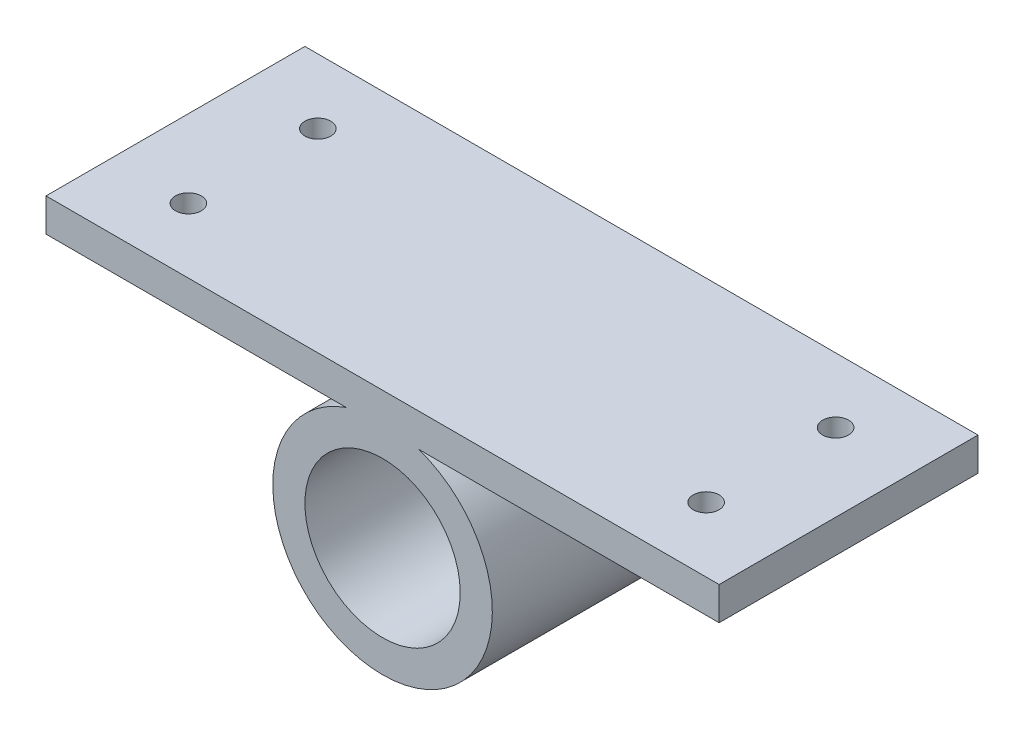
ISO-10303-21;
HEADER;
FILE_DESCRIPTION(('STEP AP214'),'2;1');
FILE_NAME('part.step','',(''),(''),'','','');
FILE_SCHEMA(('AUTOMOTIVE_DESIGN { 1 0 10303 214 1 1 1 1 }'));
ENDSEC;
DATA;
#1=APPLICATION_CONTEXT('core data for automotive mechanical design processes');
#2=APPLICATION_PROTOCOL_DEFINITION('international standard','automotive_design',2000,#1);
#3=PRODUCT_CONTEXT('',#1,'mechanical');
#4=PRODUCT('Part','Part','',(#3));
#5=PRODUCT_RELATED_PRODUCT_CATEGORY('part','',(#4));
#6=PRODUCT_DEFINITION_FORMATION('','',#4);
#7=PRODUCT_DEFINITION_CONTEXT('part definition',#1,'design');
#8=PRODUCT_DEFINITION('design','',#6,#7);
#9=PRODUCT_DEFINITION_SHAPE('','',#8);
#10=(LENGTH_UNIT() NAMED_UNIT(*) SI_UNIT(.MILLI.,.METRE.));
#11=(NAMED_UNIT(*) PLANE_ANGLE_UNIT() SI_UNIT($,.RADIAN.));
#12=(NAMED_UNIT(*) SI_UNIT($,.STERADIAN.) SOLID_ANGLE_UNIT());
#13=UNCERTAINTY_MEASURE_WITH_UNIT(LENGTH_MEASURE(1.E-05),#10,'distance_accuracy_value','');
#14=(GEOMETRIC_REPRESENTATION_CONTEXT(3) GLOBAL_UNCERTAINTY_ASSIGNED_CONTEXT((#13)) GLOBAL_UNIT_ASSIGNED_CONTEXT((#10,
#11,#12)) REPRESENTATION_CONTEXT('',''));
#15=CARTESIAN_POINT('',(0.,0.,0.));
#16=DIRECTION('',(0.,0.,1.));
#17=DIRECTION('',(1.,0.,0.));
#18=AXIS2_PLACEMENT_3D('',#15,#16,#17);
#19=CARTESIAN_POINT('',(0.,-116.,250.));
#20=DIRECTION('',(0.,0.,1.));
#21=DIRECTION('',(1.,0.,0.));
#22=AXIS2_PLACEMENT_3D('',#19,#20,#21);
#23=PLANE('',#22);
#24=DIRECTION('',(0.,1.,0.));
#25=VECTOR('',#24,1.);
#26=CARTESIAN_POINT('',(325.000000000001,-16.,250.));
#27=LINE('',#26,#25);
#28=CARTESIAN_POINT('',(325.000000000001,-16.,250.));
#29=VERTEX_POINT('',#28);
#30=CARTESIAN_POINT('',(325.000000000001,16.,250.));
#31=VERTEX_POINT('',#30);
#32=EDGE_CURVE('E131',#29,#31,#27,.T.);
#33=ORIENTED_EDGE('',*,*,#32,.T.);
#34=DIRECTION('',(-1.,0.,0.));
#35=VECTOR('',#34,1.);
#36=CARTESIAN_POINT('',(-324.999999999999,16.,250.));
#37=LINE('',#36,#35);
#38=CARTESIAN_POINT('',(-324.999999999999,16.,250.));
#39=VERTEX_POINT('',#38);
#40=EDGE_CURVE('E91',#31,#39,#37,.T.);
#41=ORIENTED_EDGE('',*,*,#40,.T.);
#42=DIRECTION('',(0.,-1.,0.));
#43=VECTOR('',#42,1.);
#44=CARTESIAN_POINT('',(-324.999999999999,-16.,250.));
#45=LINE('',#44,#43);
#46=CARTESIAN_POINT('',(-324.999999999999,-16.,250.));
#47=VERTEX_POINT('',#46);
#48=EDGE_CURVE('E106',#39,#47,#45,.T.);
#49=ORIENTED_EDGE('',*,*,#48,.T.);
#50=DIRECTION('',(1.,0.,0.));
#51=VECTOR('',#50,1.);
#52=CARTESIAN_POINT('',(-324.999999999999,-16.,250.));
#53=LINE('',#52,#51);
#54=CARTESIAN_POINT('',(-35.1567916624939,-16.,250.));
#55=VERTEX_POINT('',#54);
#56=EDGE_CURVE('E99',#47,#55,#53,.T.);
#57=ORIENTED_EDGE('',*,*,#56,.T.);
#58=CARTESIAN_POINT('',(0.,-116.,250.));
#59=DIRECTION('',(0.,0.,1.));
#60=DIRECTION('',(1.,0.,0.));
#61=AXIS2_PLACEMENT_3D('',#58,#59,#60);
#62=CIRCLE('',#61,106.);
#63=CARTESIAN_POINT('',(35.1567916624939,-16.,250.));
#64=VERTEX_POINT('',#63);
#65=EDGE_CURVE('E102',#55,#64,#62,.T.);
#66=ORIENTED_EDGE('',*,*,#65,.T.);
#67=DIRECTION('',(1.,0.,0.));
#68=VECTOR('',#67,1.);
#69=CARTESIAN_POINT('',(35.1567916624939,-16.,250.));
#70=LINE('',#69,#68);
#71=EDGE_CURVE('E57',#64,#29,#70,.T.);
#72=ORIENTED_EDGE('',*,*,#71,.T.);
#73=EDGE_LOOP('',(#33,#41,#49,#57,#66,#72));
#74=FACE_BOUND('',#73,.T.);
#75=CARTESIAN_POINT('',(0.,-116.,250.));
#76=DIRECTION('',(0.,0.,1.));
#77=DIRECTION('',(1.,0.,0.));
#78=AXIS2_PLACEMENT_3D('',#75,#76,#77);
#79=CIRCLE('',#78,75.);
#80=CARTESIAN_POINT('',(75.,-116.,250.));
#81=VERTEX_POINT('',#80);
#82=EDGE_CURVE('E126',#81,#81,#79,.T.);
#83=ORIENTED_EDGE('',*,*,#82,.F.);
#84=EDGE_LOOP('',(#83));
#85=FACE_BOUND('',#84,.T.);
#86=ADVANCED_FACE('F39',(#74,#85),#23,.T.);
#87=CARTESIAN_POINT('',(0.,-116.,0.));
#88=DIRECTION('',(0.,0.,1.));
#89=DIRECTION('',(1.,0.,0.));
#90=AXIS2_PLACEMENT_3D('',#87,#88,#89);
#91=PLANE('',#90);
#92=DIRECTION('',(0.,1.,0.));
#93=VECTOR('',#92,1.);
#94=CARTESIAN_POINT('',(325.000000000001,-16.,0.));
#95=LINE('',#94,#93);
#96=CARTESIAN_POINT('',(325.000000000001,-16.,0.));
#97=VERTEX_POINT('',#96);
#98=CARTESIAN_POINT('',(325.000000000001,16.,0.));
#99=VERTEX_POINT('',#98);
#100=EDGE_CURVE('E125',#97,#99,#95,.T.);
#101=ORIENTED_EDGE('',*,*,#100,.F.);
#102=DIRECTION('',(1.,0.,0.));
#103=VECTOR('',#102,1.);
#104=CARTESIAN_POINT('',(35.1567916624939,-16.,0.));
#105=LINE('',#104,#103);
#106=CARTESIAN_POINT('',(35.1567916624939,-16.,0.));
#107=VERTEX_POINT('',#106);
#108=EDGE_CURVE('E81',#107,#97,#105,.T.);
#109=ORIENTED_EDGE('',*,*,#108,.F.);
#110=CARTESIAN_POINT('',(0.,-116.,0.));
#111=DIRECTION('',(0.,0.,1.));
#112=DIRECTION('',(1.,0.,0.));
#113=AXIS2_PLACEMENT_3D('',#110,#111,#112);
#114=CIRCLE('',#113,106.);
#115=CARTESIAN_POINT('',(-35.1567916624939,-16.,0.));
#116=VERTEX_POINT('',#115);
#117=EDGE_CURVE('E80',#116,#107,#114,.T.);
#118=ORIENTED_EDGE('',*,*,#117,.F.);
#119=DIRECTION('',(1.,0.,0.));
#120=VECTOR('',#119,1.);
#121=CARTESIAN_POINT('',(-324.999999999999,-16.,0.));
#122=LINE('',#121,#120);
#123=CARTESIAN_POINT('',(-324.999999999999,-16.,0.));
#124=VERTEX_POINT('',#123);
#125=EDGE_CURVE('E111',#124,#116,#122,.T.);
#126=ORIENTED_EDGE('',*,*,#125,.F.);
#127=DIRECTION('',(0.,-1.,0.));
#128=VECTOR('',#127,1.);
#129=CARTESIAN_POINT('',(-324.999999999999,-16.,0.));
#130=LINE('',#129,#128);
#131=CARTESIAN_POINT('',(-324.999999999999,16.,0.));
#132=VERTEX_POINT('',#131);
#133=EDGE_CURVE('E128',#132,#124,#130,.T.);
#134=ORIENTED_EDGE('',*,*,#133,.F.);
#135=DIRECTION('',(-1.,0.,0.));
#136=VECTOR('',#135,1.);
#137=CARTESIAN_POINT('',(-324.999999999999,16.,0.));
#138=LINE('',#137,#136);
#139=EDGE_CURVE('E130',#99,#132,#138,.T.);
#140=ORIENTED_EDGE('',*,*,#139,.F.);
#141=EDGE_LOOP('',(#101,#109,#118,#126,#134,#140));
#142=FACE_BOUND('',#141,.T.);
#143=CARTESIAN_POINT('',(0.,-116.,0.));
#144=DIRECTION('',(0.,0.,1.));
#145=DIRECTION('',(1.,0.,0.));
#146=AXIS2_PLACEMENT_3D('',#143,#144,#145);
#147=CIRCLE('',#146,75.);
#148=CARTESIAN_POINT('',(75.,-116.,0.));
#149=VERTEX_POINT('',#148);
#150=EDGE_CURVE('E216',#149,#149,#147,.T.);
#151=ORIENTED_EDGE('',*,*,#150,.T.);
#152=EDGE_LOOP('',(#151));
#153=FACE_BOUND('',#152,.T.);
#154=ADVANCED_FACE('F145',(#142,#153),#91,.F.);
#155=CARTESIAN_POINT('',(325.000000000001,-16.,250.));
#156=DIRECTION('',(-1.,0.,0.));
#157=DIRECTION('',(0.,0.,1.));
#158=AXIS2_PLACEMENT_3D('',#155,#156,#157);
#159=PLANE('',#158);
#160=ORIENTED_EDGE('',*,*,#100,.T.);
#161=DIRECTION('',(0.,0.,-1.));
#162=VECTOR('',#161,1.);
#163=CARTESIAN_POINT('',(325.000000000001,16.,250.));
#164=LINE('',#163,#162);
#165=EDGE_CURVE('E11',#31,#99,#164,.T.);
#166=ORIENTED_EDGE('',*,*,#165,.F.);
#167=ORIENTED_EDGE('',*,*,#32,.F.);
#168=DIRECTION('',(0.,0.,-1.));
#169=VECTOR('',#168,1.);
#170=CARTESIAN_POINT('',(325.000000000001,-16.,250.));
#171=LINE('',#170,#169);
#172=EDGE_CURVE('E116',#29,#97,#171,.T.);
#173=ORIENTED_EDGE('',*,*,#172,.T.);
#174=EDGE_LOOP('',(#160,#166,#167,#173));
#175=FACE_BOUND('',#174,.T.);
#176=ADVANCED_FACE('F41',(#175),#159,.F.);
#177=CARTESIAN_POINT('',(-324.999999999999,16.,250.));
#178=DIRECTION('',(0.,-1.,0.));
#179=DIRECTION('',(0.,0.,-1.));
#180=AXIS2_PLACEMENT_3D('',#177,#178,#179);
#181=PLANE('',#180);
#182=CARTESIAN_POINT('',(249.999999999999,16.,62.5));
#183=DIRECTION('',(0.,1.,0.));
#184=DIRECTION('',(0.,0.,-1.));
#185=AXIS2_PLACEMENT_3D('',#182,#183,#184);
#186=CIRCLE('',#185,12.5);
#187=CARTESIAN_POINT('',(249.999999999999,16.,75.));
#188=VERTEX_POINT('',#187);
#189=EDGE_CURVE('E205',#188,#188,#186,.T.);
#190=ORIENTED_EDGE('',*,*,#189,.F.);
#191=EDGE_LOOP('',(#190));
#192=FACE_BOUND('',#191,.T.);
#193=CARTESIAN_POINT('',(-249.999999999999,16.,187.5));
#194=DIRECTION('',(0.,1.,0.));
#195=DIRECTION('',(0.,0.,1.));
#196=AXIS2_PLACEMENT_3D('',#193,#194,#195);
#197=CIRCLE('',#196,12.5);
#198=CARTESIAN_POINT('',(-249.999999999999,16.,200.));
#199=VERTEX_POINT('',#198);
#200=EDGE_CURVE('E191',#199,#199,#197,.T.);
#201=ORIENTED_EDGE('',*,*,#200,.F.);
#202=EDGE_LOOP('',(#201));
#203=FACE_BOUND('',#202,.T.);
#204=CARTESIAN_POINT('',(249.999999999999,16.,187.5));
#205=DIRECTION('',(0.,1.,0.));
#206=DIRECTION('',(0.,0.,-1.));
#207=AXIS2_PLACEMENT_3D('',#204,#205,#206);
#208=CIRCLE('',#207,12.5);
#209=CARTESIAN_POINT('',(249.999999999999,16.,200.));
#210=VERTEX_POINT('',#209);
#211=EDGE_CURVE('E193',#210,#210,#208,.T.);
#212=ORIENTED_EDGE('',*,*,#211,.F.);
#213=EDGE_LOOP('',(#212));
#214=FACE_BOUND('',#213,.T.);
#215=CARTESIAN_POINT('',(-249.999999999999,16.,62.5));
#216=DIRECTION('',(0.,1.,0.));
#217=DIRECTION('',(0.,0.,1.));
#218=AXIS2_PLACEMENT_3D('',#215,#216,#217);
#219=CIRCLE('',#218,12.5);
#220=CARTESIAN_POINT('',(-249.999999999999,16.,75.));
#221=VERTEX_POINT('',#220);
#222=EDGE_CURVE('E210',#221,#221,#219,.T.);
#223=ORIENTED_EDGE('',*,*,#222,.F.);
#224=EDGE_LOOP('',(#223));
#225=FACE_BOUND('',#224,.T.);
#226=ORIENTED_EDGE('',*,*,#139,.T.);
#227=DIRECTION('',(0.,0.,-1.));
#228=VECTOR('',#227,1.);
#229=CARTESIAN_POINT('',(-324.999999999999,16.,250.));
#230=LINE('',#229,#228);
#231=EDGE_CURVE('E48',#39,#132,#230,.T.);
#232=ORIENTED_EDGE('',*,*,#231,.F.);
#233=ORIENTED_EDGE('',*,*,#40,.F.);
#234=ORIENTED_EDGE('',*,*,#165,.T.);
#235=EDGE_LOOP('',(#226,#232,#233,#234));
#236=FACE_BOUND('',#235,.T.);
#237=ADVANCED_FACE('F235',(#192,#203,#214,#225,#236),#181,.F.);
#238=CARTESIAN_POINT('',(-324.999999999999,-16.,250.));
#239=DIRECTION('',(1.,0.,0.));
#240=DIRECTION('',(0.,0.,-1.));
#241=AXIS2_PLACEMENT_3D('',#238,#239,#240);
#242=PLANE('',#241);
#243=ORIENTED_EDGE('',*,*,#133,.T.);
#244=DIRECTION('',(0.,0.,-1.));
#245=VECTOR('',#244,1.);
#246=CARTESIAN_POINT('',(-324.999999999999,-16.,250.));
#247=LINE('',#246,#245);
#248=EDGE_CURVE('E113',#47,#124,#247,.T.);
#249=ORIENTED_EDGE('',*,*,#248,.F.);
#250=ORIENTED_EDGE('',*,*,#48,.F.);
#251=ORIENTED_EDGE('',*,*,#231,.T.);
#252=EDGE_LOOP('',(#243,#249,#250,#251));
#253=FACE_BOUND('',#252,.T.);
#254=ADVANCED_FACE('F143',(#253),#242,.F.);
#255=CARTESIAN_POINT('',(-324.999999999999,-16.,250.));
#256=DIRECTION('',(0.,1.,0.));
#257=DIRECTION('',(0.,0.,1.));
#258=AXIS2_PLACEMENT_3D('',#255,#256,#257);
#259=PLANE('',#258);
#260=CARTESIAN_POINT('',(-249.999999999999,-16.,187.5));
#261=DIRECTION('',(0.,1.,0.));
#262=DIRECTION('',(0.,0.,1.));
#263=AXIS2_PLACEMENT_3D('',#260,#261,#262);
#264=CIRCLE('',#263,12.5);
#265=CARTESIAN_POINT('',(-249.999999999999,-16.,200.));
#266=VERTEX_POINT('',#265);
#267=EDGE_CURVE('E196',#266,#266,#264,.F.);
#268=ORIENTED_EDGE('',*,*,#267,.F.);
#269=EDGE_LOOP('',(#268));
#270=FACE_BOUND('',#269,.T.);
#271=CARTESIAN_POINT('',(-249.999999999999,-16.,62.5));
#272=DIRECTION('',(0.,1.,0.));
#273=DIRECTION('',(0.,0.,1.));
#274=AXIS2_PLACEMENT_3D('',#271,#272,#273);
#275=CIRCLE('',#274,12.5);
#276=CARTESIAN_POINT('',(-249.999999999999,-16.,75.));
#277=VERTEX_POINT('',#276);
#278=EDGE_CURVE('E213',#277,#277,#275,.F.);
#279=ORIENTED_EDGE('',*,*,#278,.F.);
#280=EDGE_LOOP('',(#279));
#281=FACE_BOUND('',#280,.T.);
#282=ORIENTED_EDGE('',*,*,#125,.T.);
#283=DIRECTION('',(0.,0.,-1.));
#284=VECTOR('',#283,1.);
#285=CARTESIAN_POINT('',(-35.1567916624939,-16.,250.));
#286=LINE('',#285,#284);
#287=EDGE_CURVE('E112',#55,#116,#286,.T.);
#288=ORIENTED_EDGE('',*,*,#287,.F.);
#289=ORIENTED_EDGE('',*,*,#56,.F.);
#290=ORIENTED_EDGE('',*,*,#248,.T.);
#291=EDGE_LOOP('',(#282,#288,#289,#290));
#292=FACE_BOUND('',#291,.T.);
#293=ADVANCED_FACE('F115',(#270,#281,#292),#259,.F.);
#294=CARTESIAN_POINT('',(0.,-116.,250.));
#295=DIRECTION('',(0.,0.,-1.));
#296=DIRECTION('',(-1.,0.,0.));
#297=AXIS2_PLACEMENT_3D('',#294,#295,#296);
#298=CYLINDRICAL_SURFACE('',#297,106.);
#299=ORIENTED_EDGE('',*,*,#117,.T.);
#300=DIRECTION('',(0.,0.,-1.));
#301=VECTOR('',#300,1.);
#302=CARTESIAN_POINT('',(35.1567916624939,-16.,250.));
#303=LINE('',#302,#301);
#304=EDGE_CURVE('E118',#64,#107,#303,.T.);
#305=ORIENTED_EDGE('',*,*,#304,.F.);
#306=ORIENTED_EDGE('',*,*,#65,.F.);
#307=ORIENTED_EDGE('',*,*,#287,.T.);
#308=EDGE_LOOP('',(#299,#305,#306,#307));
#309=FACE_BOUND('',#308,.T.);
#310=ADVANCED_FACE('F117',(#309),#298,.T.);
#311=CARTESIAN_POINT('',(35.1567916624939,-16.,250.));
#312=DIRECTION('',(0.,1.,0.));
#313=DIRECTION('',(0.,0.,1.));
#314=AXIS2_PLACEMENT_3D('',#311,#312,#313);
#315=PLANE('',#314);
#316=CARTESIAN_POINT('',(249.999999999999,-16.,62.5));
#317=DIRECTION('',(0.,1.,0.));
#318=DIRECTION('',(0.,0.,1.));
#319=AXIS2_PLACEMENT_3D('',#316,#317,#318);
#320=CIRCLE('',#319,12.5);
#321=CARTESIAN_POINT('',(249.999999999999,-16.,75.));
#322=VERTEX_POINT('',#321);
#323=EDGE_CURVE('E202',#322,#322,#320,.F.);
#324=ORIENTED_EDGE('',*,*,#323,.F.);
#325=EDGE_LOOP('',(#324));
#326=FACE_BOUND('',#325,.T.);
#327=CARTESIAN_POINT('',(249.999999999999,-16.,187.5));
#328=DIRECTION('',(0.,1.,0.));
#329=DIRECTION('',(0.,0.,1.));
#330=AXIS2_PLACEMENT_3D('',#327,#328,#329);
#331=CIRCLE('',#330,12.5);
#332=CARTESIAN_POINT('',(249.999999999999,-16.,200.));
#333=VERTEX_POINT('',#332);
#334=EDGE_CURVE('E195',#333,#333,#331,.F.);
#335=ORIENTED_EDGE('',*,*,#334,.F.);
#336=EDGE_LOOP('',(#335));
#337=FACE_BOUND('',#336,.T.);
#338=ORIENTED_EDGE('',*,*,#108,.T.);
#339=ORIENTED_EDGE('',*,*,#172,.F.);
#340=ORIENTED_EDGE('',*,*,#71,.F.);
#341=ORIENTED_EDGE('',*,*,#304,.T.);
#342=EDGE_LOOP('',(#338,#339,#340,#341));
#343=FACE_BOUND('',#342,.T.);
#344=ADVANCED_FACE('F149',(#326,#337,#343),#315,.F.);
#345=CARTESIAN_POINT('',(0.,-116.,250.));
#346=DIRECTION('',(0.,0.,-1.));
#347=DIRECTION('',(-1.,0.,0.));
#348=AXIS2_PLACEMENT_3D('',#345,#346,#347);
#349=CYLINDRICAL_SURFACE('',#348,75.);
#350=ORIENTED_EDGE('',*,*,#82,.T.);
#351=EDGE_LOOP('',(#350));
#352=FACE_BOUND('',#351,.T.);
#353=ORIENTED_EDGE('',*,*,#150,.F.);
#354=EDGE_LOOP('',(#353));
#355=FACE_BOUND('',#354,.T.);
#356=ADVANCED_FACE('F151',(#352,#355),#349,.F.);
#357=CARTESIAN_POINT('',(249.999999999999,-222.001,187.5));
#358=DIRECTION('',(0.,1.,0.));
#359=DIRECTION('',(0.,0.,1.));
#360=AXIS2_PLACEMENT_3D('',#357,#358,#359);
#361=CYLINDRICAL_SURFACE('',#360,12.5);
#362=CARTESIAN_POINT('',(249.999999999999,16.,200.));
#363=CARTESIAN_POINT('',(249.999999999999,15.6666666666667,200.));
#364=CARTESIAN_POINT('',(249.999999999999,15.3333333333333,200.));
#365=CARTESIAN_POINT('',(249.999999999999,14.6666666666667,200.));
#366=CARTESIAN_POINT('',(249.999999999999,14.3333333333333,200.));
#367=CARTESIAN_POINT('',(249.999999999999,13.6666666666667,200.));
#368=CARTESIAN_POINT('',(249.999999999999,13.3333333333333,200.));
#369=CARTESIAN_POINT('',(249.999999999999,12.6666666666667,200.));
#370=CARTESIAN_POINT('',(249.999999999999,12.3333333333333,200.));
#371=CARTESIAN_POINT('',(249.999999999999,11.6666666666667,200.));
#372=CARTESIAN_POINT('',(249.999999999999,11.3333333333333,200.));
#373=CARTESIAN_POINT('',(249.999999999999,10.6666666666666,200.));
#374=CARTESIAN_POINT('',(249.999999999999,10.3333333333333,200.));
#375=CARTESIAN_POINT('',(249.999999999999,9.66666666666665,200.));
#376=CARTESIAN_POINT('',(249.999999999999,9.33333333333331,200.));
#377=CARTESIAN_POINT('',(249.999999999999,8.66666666666665,200.));
#378=CARTESIAN_POINT('',(249.999999999999,8.33333333333331,200.));
#379=CARTESIAN_POINT('',(249.999999999999,7.66666666666665,200.));
#380=CARTESIAN_POINT('',(249.999999999999,7.33333333333331,200.));
#381=CARTESIAN_POINT('',(249.999999999999,6.66666666666664,200.));
#382=CARTESIAN_POINT('',(249.999999999999,6.33333333333331,200.));
#383=CARTESIAN_POINT('',(249.999999999999,5.66666666666664,200.));
#384=CARTESIAN_POINT('',(249.999999999999,5.33333333333331,200.));
#385=CARTESIAN_POINT('',(249.999999999999,4.66666666666664,200.));
#386=CARTESIAN_POINT('',(249.999999999999,4.33333333333331,200.));
#387=CARTESIAN_POINT('',(249.999999999999,3.66666666666664,200.));
#388=CARTESIAN_POINT('',(249.999999999999,3.33333333333331,200.));
#389=CARTESIAN_POINT('',(249.999999999999,2.66666666666664,200.));
#390=CARTESIAN_POINT('',(249.999999999999,2.33333333333331,200.));
#391=CARTESIAN_POINT('',(249.999999999999,1.66666666666664,200.));
#392=CARTESIAN_POINT('',(249.999999999999,1.33333333333331,200.));
#393=CARTESIAN_POINT('',(249.999999999999,0.666666666666639,200.));
#394=CARTESIAN_POINT('',(249.999999999999,0.333333333333306,200.));
#395=CARTESIAN_POINT('',(249.999999999999,-0.333333333333361,200.));
#396=CARTESIAN_POINT('',(249.999999999999,-0.666666666666695,200.));
#397=CARTESIAN_POINT('',(249.999999999999,-1.33333333333336,200.));
#398=CARTESIAN_POINT('',(249.999999999999,-1.6666666666667,200.));
#399=CARTESIAN_POINT('',(249.999999999999,-2.33333333333336,200.));
#400=CARTESIAN_POINT('',(249.999999999999,-2.6666666666667,200.));
#401=CARTESIAN_POINT('',(249.999999999999,-3.33333333333336,200.));
#402=CARTESIAN_POINT('',(249.999999999999,-3.6666666666667,200.));
#403=CARTESIAN_POINT('',(249.999999999999,-4.33333333333337,200.));
#404=CARTESIAN_POINT('',(249.999999999999,-4.6666666666667,200.));
#405=CARTESIAN_POINT('',(249.999999999999,-5.33333333333337,200.));
#406=CARTESIAN_POINT('',(249.999999999999,-5.6666666666667,200.));
#407=CARTESIAN_POINT('',(249.999999999999,-6.33333333333337,200.));
#408=CARTESIAN_POINT('',(249.999999999999,-6.6666666666667,200.));
#409=CARTESIAN_POINT('',(249.999999999999,-7.33333333333337,200.));
#410=CARTESIAN_POINT('',(249.999999999999,-7.6666666666667,200.));
#411=CARTESIAN_POINT('',(249.999999999999,-8.33333333333337,200.));
#412=CARTESIAN_POINT('',(249.999999999999,-8.6666666666667,200.));
#413=CARTESIAN_POINT('',(249.999999999999,-9.33333333333337,200.));
#414=CARTESIAN_POINT('',(249.999999999999,-9.6666666666667,200.));
#415=CARTESIAN_POINT('',(249.999999999999,-10.3333333333334,200.));
#416=CARTESIAN_POINT('',(249.999999999999,-10.6666666666667,200.));
#417=CARTESIAN_POINT('',(249.999999999999,-11.3333333333334,200.));
#418=CARTESIAN_POINT('',(249.999999999999,-11.6666666666667,200.));
#419=CARTESIAN_POINT('',(249.999999999999,-12.3333333333334,200.));
#420=CARTESIAN_POINT('',(249.999999999999,-12.6666666666667,200.));
#421=CARTESIAN_POINT('',(249.999999999999,-13.3333333333334,200.));
#422=CARTESIAN_POINT('',(249.999999999999,-13.6666666666667,200.));
#423=CARTESIAN_POINT('',(249.999999999999,-14.3333333333334,200.));
#424=CARTESIAN_POINT('',(249.999999999999,-14.6666666666667,200.));
#425=CARTESIAN_POINT('',(249.999999999999,-15.3333333333334,200.));
#426=CARTESIAN_POINT('',(249.999999999999,-15.6666666666667,200.));
#427=CARTESIAN_POINT('',(249.999999999999,-16.,200.));
#428=B_SPLINE_CURVE_WITH_KNOTS('',3,(#362,#363,#364,#365,#366,#367,#368,#369,#370,#371,#372,
#373,#374,#375,#376,#377,#378,#379,#380,#381,#382,#383,#384,#385,#386,#387,#388,#389,#390,#391,
#392,#393,#394,#395,#396,#397,#398,#399,#400,#401,#402,#403,#404,#405,#406,#407,#408,#409,#410,
#411,#412,#413,#414,#415,#416,#417,#418,#419,#420,#421,#422,#423,#424,#425,#426,#427),
.UNSPECIFIED.,.F.,.F.,(4,2,2,2,2,2,2,2,2,2,2,2,2,2,2,2,2,2,2,2,2,2,2,2,2,2,2,2,2,2,2,2,4),(0.,
1.,2.,3.,4.,5.,6.00000000000001,7.00000000000001,8.00000000000001,9.00000000000001,10.,11.,12.,
13.,14.,15.,16.,17.,18.,19.,20.,21.,22.,23.,24.,25.,26.,27.,28.,29.,30.,31.,32.),.UNSPECIFIED.);
#429=EDGE_CURVE('BSEAM157',#210,#333,#428,.T.);
#430=ORIENTED_EDGE('',*,*,#211,.T.);
#431=ORIENTED_EDGE('',*,*,#334,.T.);
#432=ORIENTED_EDGE('',*,*,#429,.T.);
#433=ORIENTED_EDGE('',*,*,#429,.F.);
#434=EDGE_LOOP('',(#430,#432,#431,#433));
#435=FACE_BOUND('',#434,.T.);
#436=ADVANCED_FACE('F157',(#435),#361,.F.);
#437=CARTESIAN_POINT('',(249.999999999999,-222.001,62.5));
#438=DIRECTION('',(0.,1.,0.));
#439=DIRECTION('',(0.,0.,1.));
#440=AXIS2_PLACEMENT_3D('',#437,#438,#439);
#441=CYLINDRICAL_SURFACE('',#440,12.5);
#442=CARTESIAN_POINT('',(249.999999999999,16.,75.));
#443=CARTESIAN_POINT('',(249.999999999999,15.6666666666667,75.));
#444=CARTESIAN_POINT('',(249.999999999999,15.3333333333333,75.));
#445=CARTESIAN_POINT('',(249.999999999999,14.6666666666667,75.));
#446=CARTESIAN_POINT('',(249.999999999999,14.3333333333333,75.));
#447=CARTESIAN_POINT('',(249.999999999999,13.6666666666667,75.));
#448=CARTESIAN_POINT('',(249.999999999999,13.3333333333333,75.));
#449=CARTESIAN_POINT('',(249.999999999999,12.6666666666667,75.));
#450=CARTESIAN_POINT('',(249.999999999999,12.3333333333333,75.));
#451=CARTESIAN_POINT('',(249.999999999999,11.6666666666667,75.));
#452=CARTESIAN_POINT('',(249.999999999999,11.3333333333333,75.));
#453=CARTESIAN_POINT('',(249.999999999999,10.6666666666666,75.));
#454=CARTESIAN_POINT('',(249.999999999999,10.3333333333333,75.));
#455=CARTESIAN_POINT('',(249.999999999999,9.66666666666665,75.));
#456=CARTESIAN_POINT('',(249.999999999999,9.33333333333331,75.));
#457=CARTESIAN_POINT('',(249.999999999999,8.66666666666665,75.));
#458=CARTESIAN_POINT('',(249.999999999999,8.33333333333331,75.));
#459=CARTESIAN_POINT('',(249.999999999999,7.66666666666665,75.));
#460=CARTESIAN_POINT('',(249.999999999999,7.33333333333331,75.));
#461=CARTESIAN_POINT('',(249.999999999999,6.66666666666664,75.));
#462=CARTESIAN_POINT('',(249.999999999999,6.33333333333331,75.));
#463=CARTESIAN_POINT('',(249.999999999999,5.66666666666664,75.));
#464=CARTESIAN_POINT('',(249.999999999999,5.33333333333331,75.));
#465=CARTESIAN_POINT('',(249.999999999999,4.66666666666664,75.));
#466=CARTESIAN_POINT('',(249.999999999999,4.33333333333331,75.));
#467=CARTESIAN_POINT('',(249.999999999999,3.66666666666664,75.));
#468=CARTESIAN_POINT('',(249.999999999999,3.33333333333331,75.));
#469=CARTESIAN_POINT('',(249.999999999999,2.66666666666664,75.));
#470=CARTESIAN_POINT('',(249.999999999999,2.33333333333331,75.));
#471=CARTESIAN_POINT('',(249.999999999999,1.66666666666664,75.));
#472=CARTESIAN_POINT('',(249.999999999999,1.33333333333331,75.));
#473=CARTESIAN_POINT('',(249.999999999999,0.666666666666639,75.));
#474=CARTESIAN_POINT('',(249.999999999999,0.333333333333306,75.));
#475=CARTESIAN_POINT('',(249.999999999999,-0.333333333333361,75.));
#476=CARTESIAN_POINT('',(249.999999999999,-0.666666666666695,75.));
#477=CARTESIAN_POINT('',(249.999999999999,-1.33333333333336,75.));
#478=CARTESIAN_POINT('',(249.999999999999,-1.6666666666667,75.));
#479=CARTESIAN_POINT('',(249.999999999999,-2.33333333333336,75.));
#480=CARTESIAN_POINT('',(249.999999999999,-2.6666666666667,75.));
#481=CARTESIAN_POINT('',(249.999999999999,-3.33333333333336,75.));
#482=CARTESIAN_POINT('',(249.999999999999,-3.6666666666667,75.));
#483=CARTESIAN_POINT('',(249.999999999999,-4.33333333333337,75.));
#484=CARTESIAN_POINT('',(249.999999999999,-4.6666666666667,75.));
#485=CARTESIAN_POINT('',(249.999999999999,-5.33333333333337,75.));
#486=CARTESIAN_POINT('',(249.999999999999,-5.6666666666667,75.));
#487=CARTESIAN_POINT('',(249.999999999999,-6.33333333333337,75.));
#488=CARTESIAN_POINT('',(249.999999999999,-6.6666666666667,75.));
#489=CARTESIAN_POINT('',(249.999999999999,-7.33333333333337,75.));
#490=CARTESIAN_POINT('',(249.999999999999,-7.6666666666667,75.));
#491=CARTESIAN_POINT('',(249.999999999999,-8.33333333333337,75.));
#492=CARTESIAN_POINT('',(249.999999999999,-8.6666666666667,75.));
#493=CARTESIAN_POINT('',(249.999999999999,-9.33333333333337,75.));
#494=CARTESIAN_POINT('',(249.999999999999,-9.6666666666667,75.));
#495=CARTESIAN_POINT('',(249.999999999999,-10.3333333333334,75.));
#496=CARTESIAN_POINT('',(249.999999999999,-10.6666666666667,75.));
#497=CARTESIAN_POINT('',(249.999999999999,-11.3333333333334,75.));
#498=CARTESIAN_POINT('',(249.999999999999,-11.6666666666667,75.));
#499=CARTESIAN_POINT('',(249.999999999999,-12.3333333333334,75.));
#500=CARTESIAN_POINT('',(249.999999999999,-12.6666666666667,75.));
#501=CARTESIAN_POINT('',(249.999999999999,-13.3333333333334,75.));
#502=CARTESIAN_POINT('',(249.999999999999,-13.6666666666667,75.));
#503=CARTESIAN_POINT('',(249.999999999999,-14.3333333333334,75.));
#504=CARTESIAN_POINT('',(249.999999999999,-14.6666666666667,75.));
#505=CARTESIAN_POINT('',(249.999999999999,-15.3333333333334,75.));
#506=CARTESIAN_POINT('',(249.999999999999,-15.6666666666667,75.));
#507=CARTESIAN_POINT('',(249.999999999999,-16.,75.));
#508=B_SPLINE_CURVE_WITH_KNOTS('',3,(#442,#443,#444,#445,#446,#447,#448,#449,#450,#451,#452,
#453,#454,#455,#456,#457,#458,#459,#460,#461,#462,#463,#464,#465,#466,#467,#468,#469,#470,#471,
#472,#473,#474,#475,#476,#477,#478,#479,#480,#481,#482,#483,#484,#485,#486,#487,#488,#489,#490,
#491,#492,#493,#494,#495,#496,#497,#498,#499,#500,#501,#502,#503,#504,#505,#506,#507),
.UNSPECIFIED.,.F.,.F.,(4,2,2,2,2,2,2,2,2,2,2,2,2,2,2,2,2,2,2,2,2,2,2,2,2,2,2,2,2,2,2,2,4),(0.,
1.,2.,3.,4.,5.,6.00000000000001,7.00000000000001,8.00000000000001,9.00000000000001,10.,11.,12.,
13.,14.,15.,16.,17.,18.,19.,20.,21.,22.,23.,24.,25.,26.,27.,28.,29.,30.,31.,32.),.UNSPECIFIED.);
#509=EDGE_CURVE('BSEAM179',#188,#322,#508,.T.);
#510=ORIENTED_EDGE('',*,*,#189,.T.);
#511=ORIENTED_EDGE('',*,*,#323,.T.);
#512=ORIENTED_EDGE('',*,*,#509,.T.);
#513=ORIENTED_EDGE('',*,*,#509,.F.);
#514=EDGE_LOOP('',(#510,#512,#511,#513));
#515=FACE_BOUND('',#514,.T.);
#516=ADVANCED_FACE('F179',(#515),#441,.F.);
#517=CARTESIAN_POINT('',(-249.999999999999,-222.001,62.5));
#518=DIRECTION('',(0.,1.,0.));
#519=DIRECTION('',(0.,0.,1.));
#520=AXIS2_PLACEMENT_3D('',#517,#518,#519);
#521=CYLINDRICAL_SURFACE('',#520,12.5);
#522=CARTESIAN_POINT('',(-249.999999999999,16.,75.));
#523=CARTESIAN_POINT('',(-249.999999999999,15.6666666666667,75.));
#524=CARTESIAN_POINT('',(-249.999999999999,15.3333333333333,75.));
#525=CARTESIAN_POINT('',(-249.999999999999,14.6666666666667,75.));
#526=CARTESIAN_POINT('',(-249.999999999999,14.3333333333333,75.));
#527=CARTESIAN_POINT('',(-249.999999999999,13.6666666666667,75.));
#528=CARTESIAN_POINT('',(-249.999999999999,13.3333333333333,75.));
#529=CARTESIAN_POINT('',(-249.999999999999,12.6666666666667,75.));
#530=CARTESIAN_POINT('',(-249.999999999999,12.3333333333333,75.));
#531=CARTESIAN_POINT('',(-249.999999999999,11.6666666666667,75.));
#532=CARTESIAN_POINT('',(-249.999999999999,11.3333333333333,75.));
#533=CARTESIAN_POINT('',(-249.999999999999,10.6666666666666,75.));
#534=CARTESIAN_POINT('',(-249.999999999999,10.3333333333333,75.));
#535=CARTESIAN_POINT('',(-249.999999999999,9.66666666666665,75.));
#536=CARTESIAN_POINT('',(-249.999999999999,9.33333333333331,75.));
#537=CARTESIAN_POINT('',(-249.999999999999,8.66666666666665,75.));
#538=CARTESIAN_POINT('',(-249.999999999999,8.33333333333331,75.));
#539=CARTESIAN_POINT('',(-249.999999999999,7.66666666666665,75.));
#540=CARTESIAN_POINT('',(-249.999999999999,7.33333333333331,75.));
#541=CARTESIAN_POINT('',(-249.999999999999,6.66666666666664,75.));
#542=CARTESIAN_POINT('',(-249.999999999999,6.33333333333331,75.));
#543=CARTESIAN_POINT('',(-249.999999999999,5.66666666666664,75.));
#544=CARTESIAN_POINT('',(-249.999999999999,5.33333333333331,75.));
#545=CARTESIAN_POINT('',(-249.999999999999,4.66666666666664,75.));
#546=CARTESIAN_POINT('',(-249.999999999999,4.33333333333331,75.));
#547=CARTESIAN_POINT('',(-249.999999999999,3.66666666666664,75.));
#548=CARTESIAN_POINT('',(-249.999999999999,3.33333333333331,75.));
#549=CARTESIAN_POINT('',(-249.999999999999,2.66666666666664,75.));
#550=CARTESIAN_POINT('',(-249.999999999999,2.33333333333331,75.));
#551=CARTESIAN_POINT('',(-249.999999999999,1.66666666666664,75.));
#552=CARTESIAN_POINT('',(-249.999999999999,1.33333333333331,75.));
#553=CARTESIAN_POINT('',(-249.999999999999,0.666666666666639,75.));
#554=CARTESIAN_POINT('',(-249.999999999999,0.333333333333306,75.));
#555=CARTESIAN_POINT('',(-249.999999999999,-0.333333333333361,75.));
#556=CARTESIAN_POINT('',(-249.999999999999,-0.666666666666695,75.));
#557=CARTESIAN_POINT('',(-249.999999999999,-1.33333333333336,75.));
#558=CARTESIAN_POINT('',(-249.999999999999,-1.6666666666667,75.));
#559=CARTESIAN_POINT('',(-249.999999999999,-2.33333333333336,75.));
#560=CARTESIAN_POINT('',(-249.999999999999,-2.6666666666667,75.));
#561=CARTESIAN_POINT('',(-249.999999999999,-3.33333333333336,75.));
#562=CARTESIAN_POINT('',(-249.999999999999,-3.6666666666667,75.));
#563=CARTESIAN_POINT('',(-249.999999999999,-4.33333333333337,75.));
#564=CARTESIAN_POINT('',(-249.999999999999,-4.6666666666667,75.));
#565=CARTESIAN_POINT('',(-249.999999999999,-5.33333333333337,75.));
#566=CARTESIAN_POINT('',(-249.999999999999,-5.6666666666667,75.));
#567=CARTESIAN_POINT('',(-249.999999999999,-6.33333333333337,75.));
#568=CARTESIAN_POINT('',(-249.999999999999,-6.6666666666667,75.));
#569=CARTESIAN_POINT('',(-249.999999999999,-7.33333333333337,75.));
#570=CARTESIAN_POINT('',(-249.999999999999,-7.6666666666667,75.));
#571=CARTESIAN_POINT('',(-249.999999999999,-8.33333333333337,75.));
#572=CARTESIAN_POINT('',(-249.999999999999,-8.6666666666667,75.));
#573=CARTESIAN_POINT('',(-249.999999999999,-9.33333333333337,75.));
#574=CARTESIAN_POINT('',(-249.999999999999,-9.6666666666667,75.));
#575=CARTESIAN_POINT('',(-249.999999999999,-10.3333333333334,75.));
#576=CARTESIAN_POINT('',(-249.999999999999,-10.6666666666667,75.));
#577=CARTESIAN_POINT('',(-249.999999999999,-11.3333333333334,75.));
#578=CARTESIAN_POINT('',(-249.999999999999,-11.6666666666667,75.));
#579=CARTESIAN_POINT('',(-249.999999999999,-12.3333333333334,75.));
#580=CARTESIAN_POINT('',(-249.999999999999,-12.6666666666667,75.));
#581=CARTESIAN_POINT('',(-249.999999999999,-13.3333333333334,75.));
#582=CARTESIAN_POINT('',(-249.999999999999,-13.6666666666667,75.));
#583=CARTESIAN_POINT('',(-249.999999999999,-14.3333333333334,75.));
#584=CARTESIAN_POINT('',(-249.999999999999,-14.6666666666667,75.));
#585=CARTESIAN_POINT('',(-249.999999999999,-15.3333333333334,75.));
#586=CARTESIAN_POINT('',(-249.999999999999,-15.6666666666667,75.));
#587=CARTESIAN_POINT('',(-249.999999999999,-16.,75.));
#588=B_SPLINE_CURVE_WITH_KNOTS('',3,(#522,#523,#524,#525,#526,#527,#528,#529,#530,#531,#532,
#533,#534,#535,#536,#537,#538,#539,#540,#541,#542,#543,#544,#545,#546,#547,#548,#549,#550,#551,
#552,#553,#554,#555,#556,#557,#558,#559,#560,#561,#562,#563,#564,#565,#566,#567,#568,#569,#570,
#571,#572,#573,#574,#575,#576,#577,#578,#579,#580,#581,#582,#583,#584,#585,#586,#587),
.UNSPECIFIED.,.F.,.F.,(4,2,2,2,2,2,2,2,2,2,2,2,2,2,2,2,2,2,2,2,2,2,2,2,2,2,2,2,2,2,2,2,4),(0.,
1.,2.,3.,4.,5.,6.00000000000001,7.00000000000001,8.00000000000001,9.00000000000001,10.,11.,12.,
13.,14.,15.,16.,17.,18.,19.,20.,21.,22.,23.,24.,25.,26.,27.,28.,29.,30.,31.,32.),.UNSPECIFIED.);
#589=EDGE_CURVE('BSEAM172',#221,#277,#588,.T.);
#590=ORIENTED_EDGE('',*,*,#222,.T.);
#591=ORIENTED_EDGE('',*,*,#278,.T.);
#592=ORIENTED_EDGE('',*,*,#589,.T.);
#593=ORIENTED_EDGE('',*,*,#589,.F.);
#594=EDGE_LOOP('',(#590,#592,#591,#593));
#595=FACE_BOUND('',#594,.T.);
#596=ADVANCED_FACE('F172',(#595),#521,.F.);
#597=CARTESIAN_POINT('',(-249.999999999999,-222.001,187.5));
#598=DIRECTION('',(0.,1.,0.));
#599=DIRECTION('',(0.,0.,1.));
#600=AXIS2_PLACEMENT_3D('',#597,#598,#599);
#601=CYLINDRICAL_SURFACE('',#600,12.5);
#602=CARTESIAN_POINT('',(-249.999999999999,16.,200.));
#603=CARTESIAN_POINT('',(-249.999999999999,15.6666666666667,200.));
#604=CARTESIAN_POINT('',(-249.999999999999,15.3333333333333,200.));
#605=CARTESIAN_POINT('',(-249.999999999999,14.6666666666667,200.));
#606=CARTESIAN_POINT('',(-249.999999999999,14.3333333333333,200.));
#607=CARTESIAN_POINT('',(-249.999999999999,13.6666666666667,200.));
#608=CARTESIAN_POINT('',(-249.999999999999,13.3333333333333,200.));
#609=CARTESIAN_POINT('',(-249.999999999999,12.6666666666667,200.));
#610=CARTESIAN_POINT('',(-249.999999999999,12.3333333333333,200.));
#611=CARTESIAN_POINT('',(-249.999999999999,11.6666666666667,200.));
#612=CARTESIAN_POINT('',(-249.999999999999,11.3333333333333,200.));
#613=CARTESIAN_POINT('',(-249.999999999999,10.6666666666666,200.));
#614=CARTESIAN_POINT('',(-249.999999999999,10.3333333333333,200.));
#615=CARTESIAN_POINT('',(-249.999999999999,9.66666666666665,200.));
#616=CARTESIAN_POINT('',(-249.999999999999,9.33333333333331,200.));
#617=CARTESIAN_POINT('',(-249.999999999999,8.66666666666665,200.));
#618=CARTESIAN_POINT('',(-249.999999999999,8.33333333333331,200.));
#619=CARTESIAN_POINT('',(-249.999999999999,7.66666666666665,200.));
#620=CARTESIAN_POINT('',(-249.999999999999,7.33333333333331,200.));
#621=CARTESIAN_POINT('',(-249.999999999999,6.66666666666664,200.));
#622=CARTESIAN_POINT('',(-249.999999999999,6.33333333333331,200.));
#623=CARTESIAN_POINT('',(-249.999999999999,5.66666666666664,200.));
#624=CARTESIAN_POINT('',(-249.999999999999,5.33333333333331,200.));
#625=CARTESIAN_POINT('',(-249.999999999999,4.66666666666664,200.));
#626=CARTESIAN_POINT('',(-249.999999999999,4.33333333333331,200.));
#627=CARTESIAN_POINT('',(-249.999999999999,3.66666666666664,200.));
#628=CARTESIAN_POINT('',(-249.999999999999,3.33333333333331,200.));
#629=CARTESIAN_POINT('',(-249.999999999999,2.66666666666664,200.));
#630=CARTESIAN_POINT('',(-249.999999999999,2.33333333333331,200.));
#631=CARTESIAN_POINT('',(-249.999999999999,1.66666666666664,200.));
#632=CARTESIAN_POINT('',(-249.999999999999,1.33333333333331,200.));
#633=CARTESIAN_POINT('',(-249.999999999999,0.666666666666639,200.));
#634=CARTESIAN_POINT('',(-249.999999999999,0.333333333333306,200.));
#635=CARTESIAN_POINT('',(-249.999999999999,-0.333333333333361,200.));
#636=CARTESIAN_POINT('',(-249.999999999999,-0.666666666666695,200.));
#637=CARTESIAN_POINT('',(-249.999999999999,-1.33333333333336,200.));
#638=CARTESIAN_POINT('',(-249.999999999999,-1.6666666666667,200.));
#639=CARTESIAN_POINT('',(-249.999999999999,-2.33333333333336,200.));
#640=CARTESIAN_POINT('',(-249.999999999999,-2.6666666666667,200.));
#641=CARTESIAN_POINT('',(-249.999999999999,-3.33333333333336,200.));
#642=CARTESIAN_POINT('',(-249.999999999999,-3.6666666666667,200.));
#643=CARTESIAN_POINT('',(-249.999999999999,-4.33333333333337,200.));
#644=CARTESIAN_POINT('',(-249.999999999999,-4.6666666666667,200.));
#645=CARTESIAN_POINT('',(-249.999999999999,-5.33333333333337,200.));
#646=CARTESIAN_POINT('',(-249.999999999999,-5.6666666666667,200.));
#647=CARTESIAN_POINT('',(-249.999999999999,-6.33333333333337,200.));
#648=CARTESIAN_POINT('',(-249.999999999999,-6.6666666666667,200.));
#649=CARTESIAN_POINT('',(-249.999999999999,-7.33333333333337,200.));
#650=CARTESIAN_POINT('',(-249.999999999999,-7.6666666666667,200.));
#651=CARTESIAN_POINT('',(-249.999999999999,-8.33333333333337,200.));
#652=CARTESIAN_POINT('',(-249.999999999999,-8.6666666666667,200.));
#653=CARTESIAN_POINT('',(-249.999999999999,-9.33333333333337,200.));
#654=CARTESIAN_POINT('',(-249.999999999999,-9.6666666666667,200.));
#655=CARTESIAN_POINT('',(-249.999999999999,-10.3333333333334,200.));
#656=CARTESIAN_POINT('',(-249.999999999999,-10.6666666666667,200.));
#657=CARTESIAN_POINT('',(-249.999999999999,-11.3333333333334,200.));
#658=CARTESIAN_POINT('',(-249.999999999999,-11.6666666666667,200.));
#659=CARTESIAN_POINT('',(-249.999999999999,-12.3333333333334,200.));
#660=CARTESIAN_POINT('',(-249.999999999999,-12.6666666666667,200.));
#661=CARTESIAN_POINT('',(-249.999999999999,-13.3333333333334,200.));
#662=CARTESIAN_POINT('',(-249.999999999999,-13.6666666666667,200.));
#663=CARTESIAN_POINT('',(-249.999999999999,-14.3333333333334,200.));
#664=CARTESIAN_POINT('',(-249.999999999999,-14.6666666666667,200.));
#665=CARTESIAN_POINT('',(-249.999999999999,-15.3333333333334,200.));
#666=CARTESIAN_POINT('',(-249.999999999999,-15.6666666666667,200.));
#667=CARTESIAN_POINT('',(-249.999999999999,-16.,200.));
#668=B_SPLINE_CURVE_WITH_KNOTS('',3,(#602,#603,#604,#605,#606,#607,#608,#609,#610,#611,#612,
#613,#614,#615,#616,#617,#618,#619,#620,#621,#622,#623,#624,#625,#626,#627,#628,#629,#630,#631,
#632,#633,#634,#635,#636,#637,#638,#639,#640,#641,#642,#643,#644,#645,#646,#647,#648,#649,#650,
#651,#652,#653,#654,#655,#656,#657,#658,#659,#660,#661,#662,#663,#664,#665,#666,#667),
.UNSPECIFIED.,.F.,.F.,(4,2,2,2,2,2,2,2,2,2,2,2,2,2,2,2,2,2,2,2,2,2,2,2,2,2,2,2,2,2,2,2,4),(0.,
1.,2.,3.,4.,5.,6.00000000000001,7.00000000000001,8.00000000000001,9.00000000000001,10.,11.,12.,
13.,14.,15.,16.,17.,18.,19.,20.,21.,22.,23.,24.,25.,26.,27.,28.,29.,30.,31.,32.),.UNSPECIFIED.);
#669=EDGE_CURVE('BSEAM178',#199,#266,#668,.T.);
#670=ORIENTED_EDGE('',*,*,#200,.T.);
#671=ORIENTED_EDGE('',*,*,#267,.T.);
#672=ORIENTED_EDGE('',*,*,#669,.T.);
#673=ORIENTED_EDGE('',*,*,#669,.F.);
#674=EDGE_LOOP('',(#670,#672,#671,#673));
#675=FACE_BOUND('',#674,.T.);
#676=ADVANCED_FACE('F178',(#675),#601,.F.);
#677=CLOSED_SHELL('',(#86,#154,#176,#237,#254,#293,#310,#344,#356,#436,#516,#596,#676));
#678=MANIFOLD_SOLID_BREP('B2',#677);
#679=ADVANCED_BREP_SHAPE_REPRESENTATION('',(#18,#678),#14);
#680=SHAPE_DEFINITION_REPRESENTATION(#9,#679);
ENDSEC;
END-ISO-10303-21;
